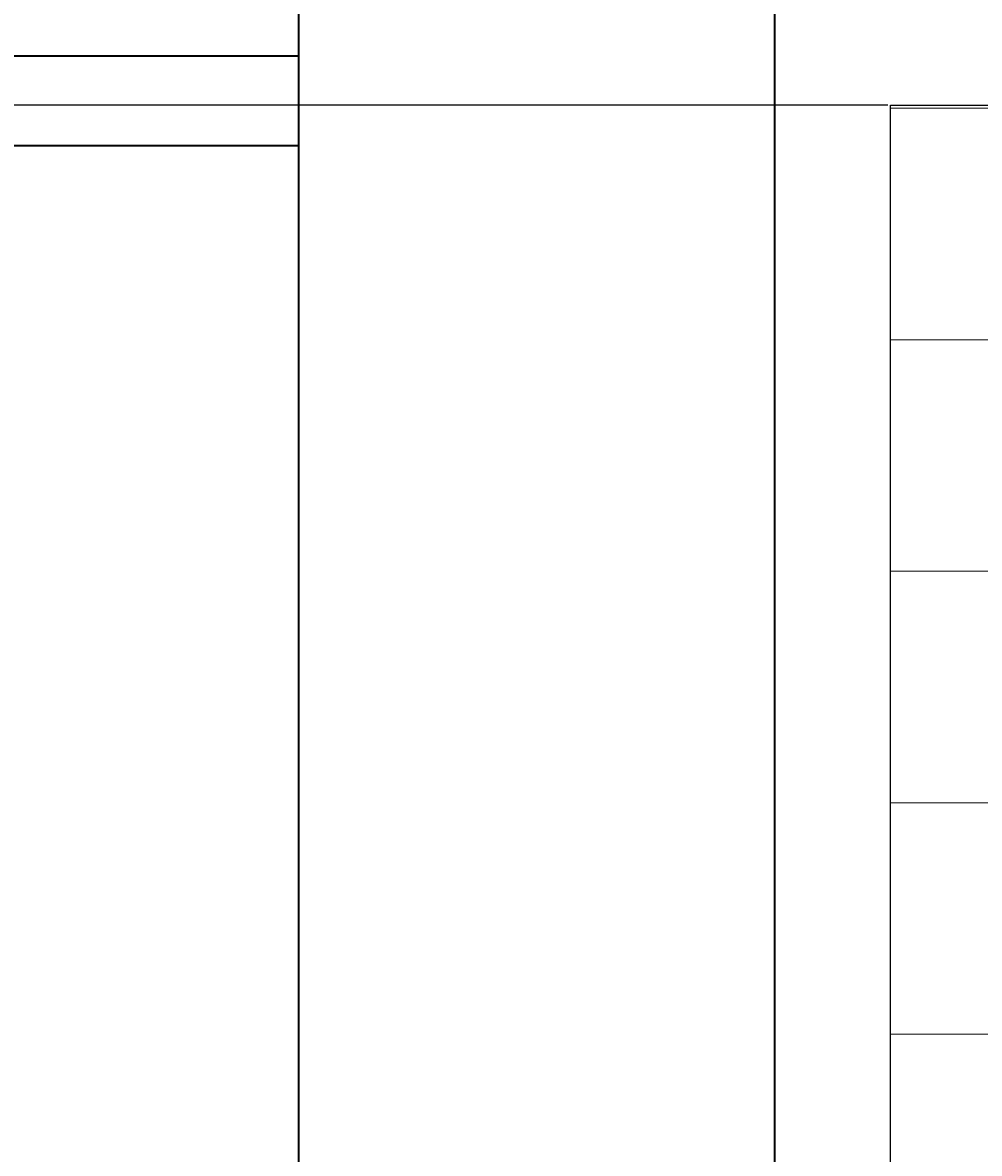
# Model space of a CAD drawing. Units: inches. Extents: x -6 to 289, y -8 to 323.
# Tile 15 of 107: x 102 to 126, y 21 to 50. Entities that reach past the tile are written whole.
import ezdxf

# ---------------------------------------------------------------- set-up
doc = ezdxf.new("R2010")
doc.units = ezdxf.units.IN
doc.header["$MEASUREMENT"] = 0
for name, color, linetype, lineweight in [('A-ANNO-DIMS', 2, 'Continuous', 18), ('A-DOOR', 3, 'Continuous', 25), ('A-ELEV', 7, 'Continuous', 35), ('A-ELEV-PATT', 8, 'Continuous', 13)]:
    doc.layers.add(name, color=color, linetype=linetype, lineweight=lineweight)
doc.styles.get("Standard").update_dxf_attribs({"font": 'arial.ttf'})
doc.dimstyles.get("Standard").update_dxf_attribs({"dimtxt": 0.18, "dimasz": 0.18, "dimexe": 0.18, "dimexo": 0.0625, "dimgap": 0.09, "dimtad": 0, "dimtih": 1, "dimtoh": 1, "dimdec": 4, "dimzin": 0, "dimdsep": 46, "dimtxsty": 'Standard', "dimcen": 0.09, "dimadec": 0, "dimazin": 0, "dimtfac": 1, "dimtdec": 4, "dimtofl": 0, "dimtmove": 0, "dimatfit": 3, "dimfxl": 1, "dimtolj": 1, "dimtzin": 0, "dimarcsym": 0})

# ---------------------------------------------------------------- blocks, each defined once
blk = doc.blocks.new('*D16')
at = {"layer": 'A-ANNO-DIMS', "color": 0, "lineweight": -2, "transparency": 16777216}
for p, q in [((9.943, 68.37), (9.943, -8.391)), ((272.973, 68.37), (272.973, -8.391)), ((10.123, -8.211), (140.993, -8.211)), ((272.793, -8.211), (141.923, -8.211))]:
    blk.add_line(p, q, dxfattribs=at)
at = {"layer": 'A-ANNO-DIMS', "color": 0, "transparency": 16777216}
for points in [[(10.123, -8.181), (10.123, -8.241), (9.943, -8.211)], [(272.793, -8.181), (272.793, -8.241), (272.973, -8.211)]]:
    blk.add_solid(points, dxfattribs=at)
at = {"layer": 'Defpoints', "color": 0, "transparency": 16777216}
for p in [(9.943, 68.432), (272.973, 68.432), (272.973, -8.211)]:
    blk.add_point(p, dxfattribs=at)
at = {"layer": 'A-ANNO-DIMS', "color": 0, "transparency": 16777216, "insert": (141.458, -8.211), "char_height": 0.18, "attachment_point": 5}
blk.add_mtext('\\A1;263.03', dxfattribs=at)
blk = doc.blocks.new('*D84')
at = {"layer": 'A-ANNO-DIMS', "color": 0, "lineweight": -2, "transparency": 16777216}
for p, q in [((123.945, 48.085), (-5.737, 48.085)), ((-5.557, 47.905), (-5.557, 29.369)), ((-5.557, 10.469), (-5.557, 29.005)), ((123.945, 10.289), (-5.737, 10.289))]:
    blk.add_line(p, q, dxfattribs=at)
at = {"layer": 'A-ANNO-DIMS', "color": 0, "transparency": 16777216}
for points in [[(-5.587, 47.905), (-5.527, 47.905), (-5.557, 48.085)], [(-5.587, 10.469), (-5.527, 10.469), (-5.557, 10.289)]]:
    blk.add_solid(points, dxfattribs=at)
at = {"layer": 'Defpoints', "color": 0, "transparency": 16777216}
for p in [(-5.557, 48.085), (124.008, 48.085), (124.008, 10.289)]:
    blk.add_point(p, dxfattribs=at)
at = {"layer": 'A-ANNO-DIMS', "color": 0, "transparency": 16777216, "insert": (-5.557, 29.187), "char_height": 0.18, "attachment_point": 5}
blk.add_mtext('\\A1;37.8', dxfattribs=at)
blk = doc.blocks.new('*D85')
at = {"layer": 'A-ANNO-DIMS', "color": 0, "lineweight": -2, "transparency": 16777216}
for p, q in [((120.945, 51.085), (-5.737, 51.085)), ((-5.557, 50.905), (-5.557, 49.767)), ((-5.557, 48.265), (-5.557, 49.403)), ((123.945, 48.085), (-5.737, 48.085))]:
    blk.add_line(p, q, dxfattribs=at)
at = {"layer": 'A-ANNO-DIMS', "color": 0, "transparency": 16777216}
for points in [[(-5.587, 50.905), (-5.527, 50.905), (-5.557, 51.085)], [(-5.587, 48.265), (-5.527, 48.265), (-5.557, 48.085)]]:
    blk.add_solid(points, dxfattribs=at)
at = {"layer": 'Defpoints', "color": 0, "transparency": 16777216}
for p in [(-5.557, 51.085), (121.008, 51.085), (124.008, 48.085)]:
    blk.add_point(p, dxfattribs=at)
at = {"layer": 'A-ANNO-DIMS', "color": 0, "transparency": 16777216, "insert": (-5.557, 49.585), "char_height": 0.18, "attachment_point": 5}
blk.add_mtext('\\A1;3', dxfattribs=at)

msp = doc.modelspace()

# ---------------------------------------------------------------- hatches: boundary and pattern name
at = {"layer": 'A-ELEV-PATT'}
h = msp.add_hatch(dxfattribs=at)
h.set_pattern_fill('_USER', color=256, scale=6, pattern_type=0)
h.set_pattern_definition([(0, (0, 0), (0, 6), [])])
h.paths.add_polyline_path([(184.1244, 48.0851), (124.008, 48.0851), (124.008, 10.2888), (184.1244, 10.2888)])
h.paths.add_polyline_path([(244.2408, 48.0851), (186.3604, 48.0851), (186.3604, 10.2888), (244.2408, 10.2888)])
h.paths.add_polyline_path([(208.2918, 114.2795), (190.7918, 114.2795), (190.7918, 71.2795), (208.2918, 71.2795)])
h.paths.add_polyline_path([(227.7918, 114.2795), (209.2918, 114.2795), (209.2918, 71.2795), (227.7918, 71.2795)])
h.paths.add_polyline_path([(211.2918, 224.3887), (190.7918, 224.3887), (190.7918, 162.3484), (211.2918, 162.3484)])
h.paths.add_polyline_path([(233.7918, 224.3887), (212.2918, 224.3887), (212.2918, 162.3484), (233.7918, 162.3484)])
h.paths.add_polyline_path([(166.3835, 224.154), (147.8835, 224.154), (147.8835, 181.154), (166.3835, 181.154)])
h.paths.add_polyline_path([(146.8835, 224.154), (129.3835, 224.154), (129.3835, 181.154), (146.8835, 181.154)])

# ---------------------------------------------------------------- linework, layer by layer
at = {"layer": 'A-DOOR'}
for points in [[(121.008, 51.0851), (247.2408, 51.0851), (247.2408, 7.2888), (121.008, 7.2888)], [(124.008, 48.0851), (244.2408, 48.0851), (244.2408, 10.2888), (124.008, 10.2888)]]:
    msp.add_lwpolyline(points, close=True, dxfattribs=at)
at = {"layer": 'A-ELEV'}
msp.add_lwpolyline([(108.6602, 66.2238), (108.6602, 7.2888), (121.008, 7.2888), (121.008, 66.2238)], dxfattribs=at)
for points in [[(24.317, 49.3604), (108.6602, 49.3604), (108.6602, 7.2888), (24.317, 7.2888)], [(24.317, 49.3604), (108.6602, 49.3604), (108.6602, 47.0304), (24.317, 47.0304)]]:
    msp.add_lwpolyline(points, close=True, dxfattribs=at)

# ---------------------------------------------------------------- dimensions: what is measured, and where the dimension line sits
at = {"layer": 'A-ANNO-DIMS'}
dim = msp.add_linear_dim(base=(272.9733, -8.2112), p1=(9.943, 68.4322), p2=(272.9733, 68.4322), dimstyle='Standard', override={"dimdec": 2, "dimlfac": 1, "dimrnd": 0, "dimzin": 0, "dimdsep": 46, "dimlunit": 2}, dxfattribs=at)
dim.commit()
dim.dimension.update_dxf_attribs({"geometry": '*D16', "text_midpoint": (141.4581, -8.2112)})
for base, p1, p2, override, picture, middle in [((-5.557, 51.0851), (124.008, 48.0851), (121.008, 51.0851), {"dimdec": 0, "dimlfac": 1, "dimrnd": 0, "dimzin": 0, "dimdsep": 46, "dimlunit": 2}, '*D85', (-5.557, 49.5851)), ((-5.557, 48.0851), (124.008, 10.2888), (124.008, 48.0851), {"dimdec": 1, "dimlfac": 1, "dimrnd": 0, "dimzin": 0, "dimdsep": 46, "dimlunit": 2}, '*D84', (-5.557, 29.187))]:
    dim = msp.add_linear_dim(base=base, p1=p1, p2=p2, angle=90, dimstyle='Standard', override=override, dxfattribs=at)
    dim.commit()
    dim.dimension.update_dxf_attribs({"geometry": picture, "text_midpoint": middle})

doc.saveas('drawing.dxf')
